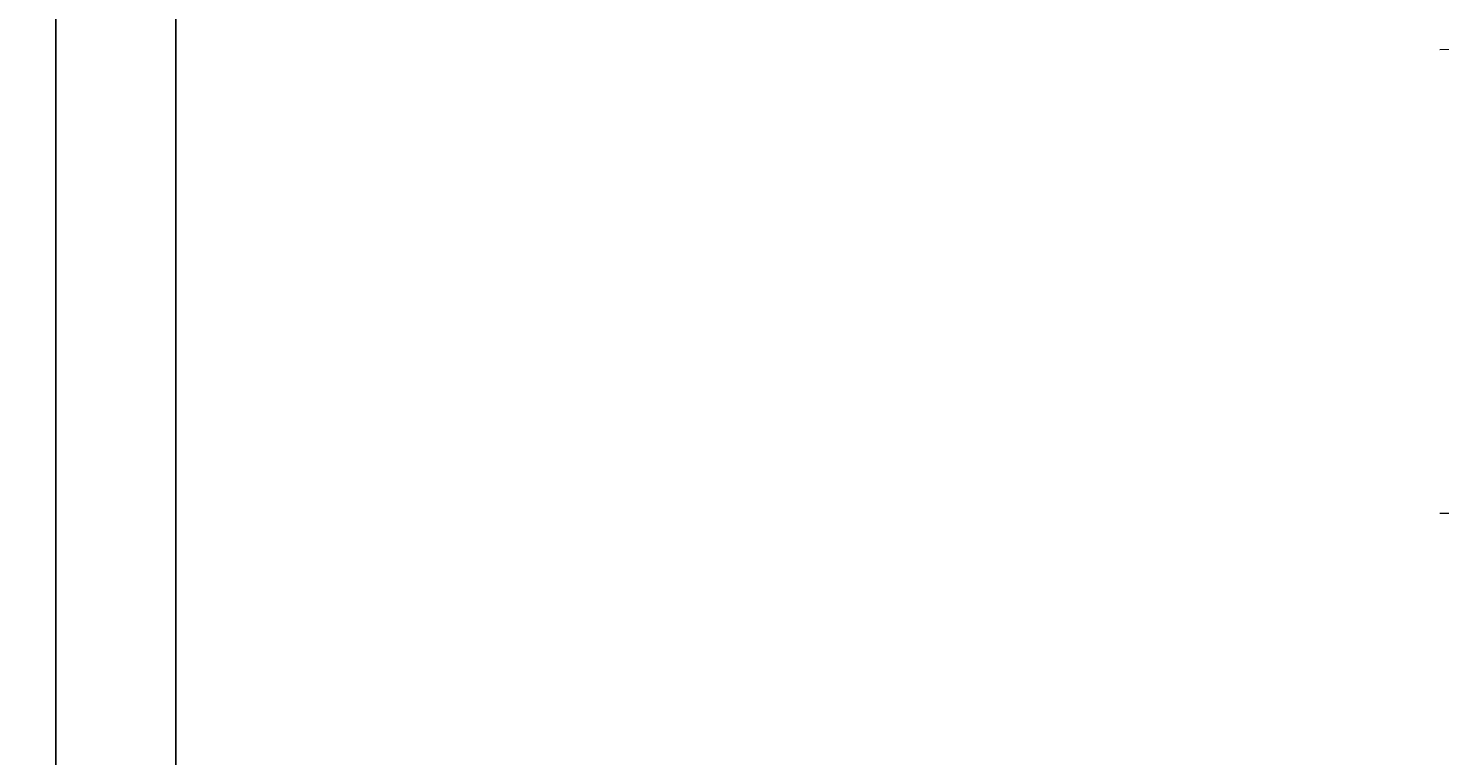
# Model space of a CAD drawing. Units: inches. Extents: x -26 to 776, y -22 to 650.
# Tile 31 of 62: x 80 to 192, y 535 to 593. Entities that reach past the tile are written whole.
import ezdxf

# ---------------------------------------------------------------- set-up
doc = ezdxf.new("R2010")
doc.units = ezdxf.units.IN
doc.header["$MEASUREMENT"] = 0
doc.layers.add('A-ANNO-DIMS', color=2, linetype='Continuous', lineweight=18)
doc.layers.add('A-WALL-TRIM', color=7, linetype='Continuous', lineweight=18)
doc.styles.get("Standard").update_dxf_attribs({"font": 'arial.ttf'})
doc.dimstyles.get("Standard").update_dxf_attribs({"dimtxt": 0.5625, "dimasz": 0.18, "dimexe": 0.18, "dimexo": 0.0625, "dimgap": 0.09, "dimtad": 0, "dimtih": 1, "dimtoh": 1, "dimdec": 4, "dimzin": 0, "dimdsep": 46, "dimlunit": 4, "dimtxsty": 'Standard', "dimcen": 0.09, "dimadec": 0, "dimazin": 0, "dimtfac": 1, "dimtdec": 4, "dimtofl": 0, "dimtmove": 0, "dimatfit": 3, "dimfxl": 1, "dimtolj": 1, "dimtzin": 0, "dimarcsym": 0})

# ---------------------------------------------------------------- blocks, each defined once
blk = doc.blocks.new('*D14')
at = {"layer": 'A-ANNO-DIMS', "color": 0, "lineweight": -2, "transparency": 16777216}
for p, q in [((191.62, 613.27), (-25.48, 613.27)), ((-25.3, 613.09), (-25.3, 314.75)), ((-25.3, 15.66), (-25.3, 314)), ((11.04, 15.48), (-25.48, 15.48))]:
    blk.add_line(p, q, dxfattribs=at)
at = {"layer": 'A-ANNO-DIMS', "color": 0, "transparency": 16777216}
for points in [[(-25.33, 613.09), (-25.27, 613.09), (-25.3, 613.27)], [(-25.33, 15.66), (-25.27, 15.66), (-25.3, 15.48)]]:
    blk.add_solid(points, dxfattribs=at)
at = {"layer": 'Defpoints', "color": 0, "transparency": 16777216}
for p in [(-25.3, 613.27), (191.68, 613.27), (11.11, 15.48)]:
    blk.add_point(p, dxfattribs=at)
at = {"layer": 'A-ANNO-DIMS', "color": 0, "transparency": 16777216, "insert": (-25.3, 314.38), "char_height": 0.562, "attachment_point": 5}
blk.add_mtext('\\A1;597.8', dxfattribs=at)
blk = doc.blocks.new('*D15')
at = {"layer": 'A-ANNO-DIMS', "color": 0, "lineweight": -2, "transparency": 16777216}
for p, q in [((11.11, 491.49), (11.11, 649.86)), ((11.29, 649.68), (120.22, 649.68)), ((231.24, 649.68), (122.31, 649.68)), ((231.42, 491.49), (231.42, 649.86))]:
    blk.add_line(p, q, dxfattribs=at)
at = {"layer": 'A-ANNO-DIMS', "color": 0, "transparency": 16777216}
for points in [[(11.29, 649.71), (11.29, 649.65), (11.11, 649.68)], [(231.24, 649.71), (231.24, 649.65), (231.42, 649.68)]]:
    blk.add_solid(points, dxfattribs=at)
at = {"layer": 'Defpoints', "color": 0, "transparency": 16777216}
for p in [(231.42, 649.68), (11.11, 491.43), (231.42, 491.43)]:
    blk.add_point(p, dxfattribs=at)
at = {"layer": 'A-ANNO-DIMS', "color": 0, "transparency": 16777216, "insert": (121.27, 649.68), "char_height": 0.562, "attachment_point": 5}
blk.add_mtext('\\A1;220.3', dxfattribs=at)
blk = doc.blocks.new('*D17')
at = {"layer": 'A-ANNO-DIMS', "color": 0, "lineweight": -2, "transparency": 16777216}
for p, q in [((11.11, 491.49), (11.11, 649.86)), ((11.29, 649.68), (100.16, 649.68)), ((191.5, 649.68), (102.62, 649.68)), ((191.68, 613.33), (191.68, 649.86))]:
    blk.add_line(p, q, dxfattribs=at)
at = {"layer": 'A-ANNO-DIMS', "color": 0, "transparency": 16777216}
for points in [[(11.29, 649.71), (11.29, 649.65), (11.11, 649.68)], [(191.5, 649.71), (191.5, 649.65), (191.68, 649.68)]]:
    blk.add_solid(points, dxfattribs=at)
at = {"layer": 'Defpoints', "color": 0, "transparency": 16777216}
for p in [(191.68, 649.68), (191.68, 613.27), (11.11, 491.43)]:
    blk.add_point(p, dxfattribs=at)
at = {"layer": 'A-ANNO-DIMS', "color": 0, "transparency": 16777216, "insert": (101.39, 649.68), "char_height": 0.562, "attachment_point": 5}
blk.add_mtext('\\A1;180.57', dxfattribs=at)
blk = doc.blocks.new('*D19')
at = {"layer": 'A-ANNO-DIMS', "color": 0, "lineweight": -2, "transparency": 16777216}
for p, q in [((191.62, 613.27), (-25.48, 613.27)), ((-25.3, 613.09), (-25.3, 552.73)), ((-25.3, 491.61), (-25.3, 551.97)), ((191.62, 491.43), (-25.48, 491.43))]:
    blk.add_line(p, q, dxfattribs=at)
at = {"layer": 'A-ANNO-DIMS', "color": 0, "transparency": 16777216}
for points in [[(-25.33, 613.09), (-25.27, 613.09), (-25.3, 613.27)], [(-25.33, 491.61), (-25.27, 491.61), (-25.3, 491.43)]]:
    blk.add_solid(points, dxfattribs=at)
at = {"layer": 'Defpoints', "color": 0, "transparency": 16777216}
for p in [(-25.3, 613.27), (191.68, 613.27), (191.68, 491.43)]:
    blk.add_point(p, dxfattribs=at)
at = {"layer": 'A-ANNO-DIMS', "color": 0, "transparency": 16777216, "insert": (-25.3, 552.35), "char_height": 0.562, "attachment_point": 5}
blk.add_mtext('\\A1;121.84', dxfattribs=at)
blk = doc.blocks.new('*D22')
at = {"layer": 'A-ANNO-DIMS', "color": 0, "lineweight": -2, "transparency": 16777216}
for p, q in [((22.89, 15.33), (22.89, 649.86)), ((23.07, 649.68), (119.19, 649.68)), ((217.77, 649.68), (121.65, 649.68)), ((217.95, 15.54), (217.95, 649.86))]:
    blk.add_line(p, q, dxfattribs=at)
at = {"layer": 'A-ANNO-DIMS', "color": 0, "transparency": 16777216}
for points in [[(23.07, 649.71), (23.07, 649.65), (22.89, 649.68)], [(217.77, 649.71), (217.77, 649.65), (217.95, 649.68)]]:
    blk.add_solid(points, dxfattribs=at)
at = {"layer": 'Defpoints', "color": 0, "transparency": 16777216}
for p in [(217.95, 649.68), (22.89, 15.27), (217.95, 15.48)]:
    blk.add_point(p, dxfattribs=at)
at = {"layer": 'A-ANNO-DIMS', "color": 0, "transparency": 16777216, "insert": (120.42, 649.68), "char_height": 0.562, "attachment_point": 5}
blk.add_mtext('\\A1;195.06', dxfattribs=at)
blk = doc.blocks.new('*D25')
at = {"layer": 'A-ANNO-DIMS', "color": 0, "lineweight": -2, "transparency": 16777216}
for p, q in [((11.11, 221.7), (11.11, 649.86)), ((11.29, 649.68), (50.34, 649.68)), ((91.46, 649.68), (52.41, 649.68)), ((91.64, 271.37), (91.64, 649.86))]:
    blk.add_line(p, q, dxfattribs=at)
at = {"layer": 'A-ANNO-DIMS', "color": 0, "transparency": 16777216}
for points in [[(11.29, 649.71), (11.29, 649.65), (11.11, 649.68)], [(91.46, 649.71), (91.46, 649.65), (91.64, 649.68)]]:
    blk.add_solid(points, dxfattribs=at)
at = {"layer": 'Defpoints', "color": 0, "transparency": 16777216}
for p in [(91.64, 649.68), (91.64, 271.31), (11.11, 221.64)]:
    blk.add_point(p, dxfattribs=at)
at = {"layer": 'A-ANNO-DIMS', "color": 0, "transparency": 16777216, "insert": (51.38, 649.68), "char_height": 0.562, "attachment_point": 5}
blk.add_mtext('\\A1;80.54', dxfattribs=at)
blk = doc.blocks.new('*D35')
at = {"layer": 'A-ANNO-DIMS', "color": 0, "lineweight": -2, "transparency": 16777216}
for p, q in [((82.13, 420.34), (82.13, 649.86)), ((82.31, 649.68), (144.38, 649.68)), ((208.91, 649.68), (146.84, 649.68)), ((209.09, 420.34), (209.09, 649.86))]:
    blk.add_line(p, q, dxfattribs=at)
at = {"layer": 'A-ANNO-DIMS', "color": 0, "transparency": 16777216}
for points in [[(82.31, 649.71), (82.31, 649.65), (82.13, 649.68)], [(208.91, 649.71), (208.91, 649.65), (209.09, 649.68)]]:
    blk.add_solid(points, dxfattribs=at)
at = {"layer": 'Defpoints', "color": 0, "transparency": 16777216}
for p in [(209.09, 649.68), (82.13, 420.28), (209.09, 420.28)]:
    blk.add_point(p, dxfattribs=at)
at = {"layer": 'A-ANNO-DIMS', "color": 0, "transparency": 16777216, "insert": (145.61, 649.68), "char_height": 0.562, "attachment_point": 5}
blk.add_mtext('\\A1;126.96', dxfattribs=at)

msp = doc.modelspace()

# ---------------------------------------------------------------- linework, layer by layer
at = {"layer": 'A-WALL-TRIM'}
for p, q in [((191.6719, 591.0323), (357.2511, 591.5545)), ((191.6719, 554.3491), (357.2511, 554.8713))]:
    msp.add_line(p, q, dxfattribs=at)

# ---------------------------------------------------------------- dimensions: what is measured, and where the dimension line sits
at = {"layer": 'A-ANNO-DIMS'}
for base, p1, p2, override, picture, middle in [((231.4249, 649.6763), (11.1074, 491.4269), (231.4249, 491.4269), {"dimdec": 1, "dimlfac": 1, "dimrnd": 0, "dimzin": 0, "dimdsep": 46, "dimlunit": 2}, '*D15', (121.2661, 649.6763)), ((191.6782, 649.6763), (11.1074, 491.4269), (191.6782, 613.2713), {"dimdec": 2, "dimlfac": 1, "dimrnd": 0, "dimzin": 0, "dimdsep": 46, "dimlunit": 2}, '*D17', (101.3928, 649.6763)), ((91.6448, 649.6763), (11.1074, 221.6413), (91.6448, 271.3091), {"dimdec": 2, "dimlfac": 1, "dimrnd": 0, "dimzin": 0, "dimdsep": 46, "dimlunit": 2}, '*D25', (51.3761, 649.6763)), ((217.9529, 649.6763), (22.8891, 15.2701), (217.9529, 15.4824), {"dimdec": 2, "dimlfac": 1, "dimrnd": 0, "dimzin": 0, "dimdsep": 46, "dimlunit": 2}, '*D22', (120.421, 649.6763)), ((209.091, 649.6763), (82.134, 420.2783), (209.091, 420.2783), {"dimdec": 2, "dimlfac": 1, "dimrnd": 0, "dimzin": 0, "dimdsep": 46, "dimlunit": 2}, '*D35', (145.6125, 649.6763))]:
    dim = msp.add_linear_dim(base=base, p1=p1, p2=p2, dimstyle='Standard', override=override, dxfattribs=at)
    dim.commit()
    dim.dimension.update_dxf_attribs({"geometry": picture, "text_midpoint": middle})
for p1, override, picture, middle in [((191.6782, 491.4269), {"dimdec": 2, "dimlfac": 1, "dimrnd": 0, "dimzin": 0, "dimdsep": 46, "dimlunit": 2}, '*D19', (-25.2976, 552.3491)), ((11.1074, 15.4824), {"dimdec": 1, "dimlfac": 1, "dimrnd": 0, "dimzin": 0, "dimdsep": 46, "dimlunit": 2}, '*D14', (-25.2976, 314.3769))]:
    dim = msp.add_linear_dim(base=(-25.2976, 613.2713), p1=p1, p2=(191.6782, 613.2713), angle=90, dimstyle='Standard', override=override, dxfattribs=at)
    dim.commit()
    dim.dimension.update_dxf_attribs({"geometry": picture, "text_midpoint": middle})

doc.saveas('drawing.dxf')
